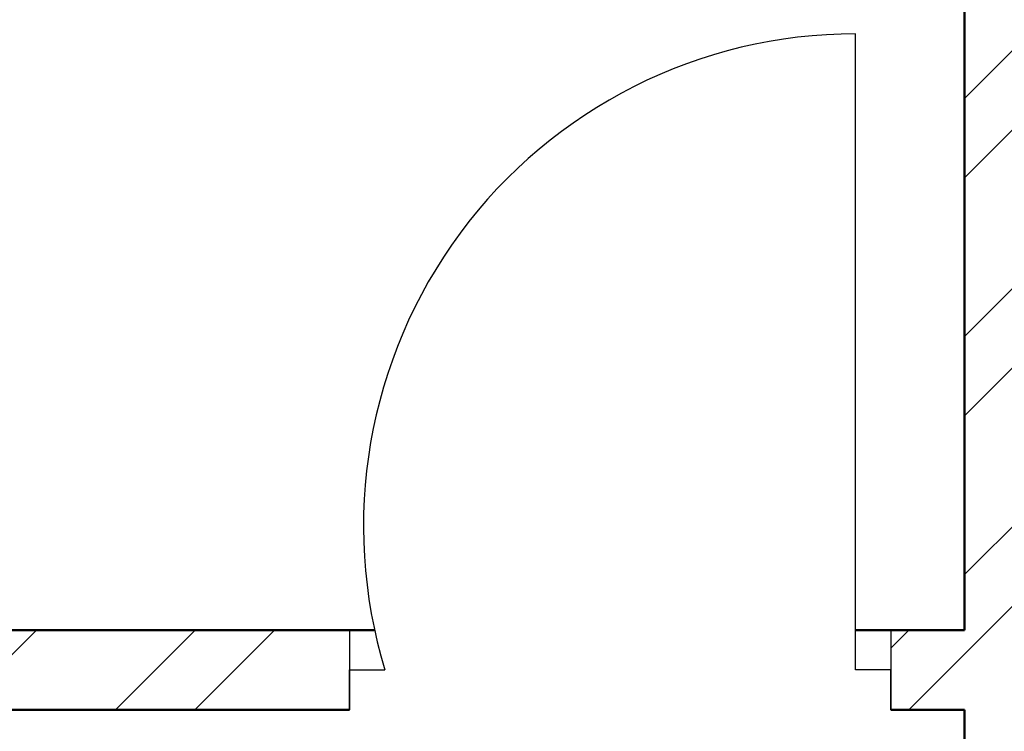
# Model space of a CAD drawing. Units: inches. Extents: x 963 to 2075, y 289 to 2657.
# Tile 70 of 98: x 1455 to 1511, y 2160 to 2200. Entities that reach past the tile are written whole.
import ezdxf

# ---------------------------------------------------------------- set-up
doc = ezdxf.new("R2010")
doc.units = ezdxf.units.IN
for name, color, linetype, lineweight in [('A-DOOR', 4, 'Continuous', 25), ('A-WALL', 7, 'Continuous', 50), ('A-WALL-PATT', 8, 'Continuous', 13)]:
    doc.layers.add(name, color=color, linetype=linetype, lineweight=lineweight)

msp = doc.modelspace()

# ---------------------------------------------------------------- hatches: boundary and pattern name
at = {"layer": 'A-WALL-PATT'}
h = msp.add_hatch(dxfattribs=at)
h.set_pattern_fill('ANSI32', color=256)
h.paths.add_polyline_path([(1296.922, 2558.318), (1203.922, 2558.318), (1203.922, 2493.818), (1191.533, 2493.818), (1191.533, 2489.318), (1211.063, 2489.318), (1211.063, 2492.02), (1211.063, 2493.818), (1208.422, 2493.818), (1208.422, 2553.818), (1292.422, 2553.818), (1292.422, 2538.863), (1296.922, 2538.863)])
h.paths.add_polyline_path([(1442.422, 2558.318), (1349.422, 2558.318), (1349.422, 2538.943), (1353.922, 2538.943), (1353.922, 2553.818), (1437.922, 2553.818), (1437.922, 2493.818), (1434.542, 2493.818), (1434.542, 2489.318), (1448.311, 2489.318), (1448.311, 2491.568), (1448.311, 2493.818), (1442.422, 2493.818)])
h.paths.add_polyline_path([(1415.554, 2491.568), (1415.554, 2493.818), (1340.941, 2493.818), (1340.941, 2489.318), (1371.922, 2489.318), (1371.922, 2378.318), (1367.596, 2378.318), (1367.596, 2373.818), (1371.922, 2373.818), (1371.922, 2355.185), (1376.422, 2355.185), (1376.422, 2489.318), (1415.554, 2489.318)])
h.paths.add_polyline_path([(1304.941, 2491.568), (1304.941, 2493.818), (1296.922, 2493.818), (1296.922, 2514.863), (1292.422, 2514.863), (1292.422, 2493.818), (1232.808, 2493.818), (1232.808, 2489.318), (1256.422, 2489.318), (1256.422, 2327.318), (1253.714, 2327.318), (1253.714, 2322.818), (1328.422, 2322.818), (1328.422, 2331.147), (1323.922, 2331.147), (1323.922, 2327.318), (1260.922, 2327.318), (1260.922, 2373.818), (1323.922, 2373.818), (1323.922, 2357.812), (1328.422, 2357.812), (1328.422, 2373.818), (1346.007, 2373.818), (1346.007, 2376.068), (1346.007, 2378.318), (1260.922, 2378.318), (1260.922, 2489.318), (1304.941, 2489.318)])
h.paths.add_polyline_path([(1226.654, 2327.318), (1124.422, 2327.318), (1124.422, 2347.447), (1119.922, 2347.447), (1119.922, 2322.818), (1163.422, 2322.818), (1163.422, 2305.435), (1165.672, 2305.435), (1167.922, 2305.435), (1167.922, 2322.818), (1226.654, 2322.818), (1226.654, 2325.068)])
h.paths.add_polyline_path([(1095.922, 2489.318), (1124.422, 2489.318), (1131.533, 2489.318), (1131.533, 2491.568), (1131.533, 2493.818), (1119.922, 2493.818), (1091.422, 2493.818), (1091.422, 2417.318), (1095.922, 2417.318), (1119.922, 2417.318), (1119.922, 2407.447), (1124.422, 2407.447), (1124.422, 2421.818), (1095.922, 2421.818)])
h.paths.add_polyline_path([(1512.922, 2558.318), (1508.422, 2558.318), (1508.422, 2493.818), (1503.401, 2493.818), (1503.401, 2489.318), (1508.422, 2489.318), (1508.422, 2327.318), (1376.422, 2327.318), (1376.422, 2330.273), (1371.922, 2330.273), (1371.922, 2298.744), (1376.422, 2298.744), (1376.422, 2322.818), (1508.422, 2322.818), (1508.422, 2165.318), (1504.255, 2165.318), (1504.255, 2160.818), (1508.422, 2160.818), (1508.422, 2108.318), (1512.922, 2108.318), (1512.922, 2160.818), (1516.182, 2160.818), (1516.182, 2163.068), (1516.182, 2165.318), (1512.922, 2165.318), (1512.922, 2322.818), (1644.922, 2322.818), (1644.922, 2298.744), (1649.422, 2298.744), (1649.422, 2322.818), (1649.422, 2330.944), (1647.172, 2330.944), (1644.922, 2330.944), (1644.922, 2327.318), (1512.922, 2327.318), (1512.922, 2489.318), (1516.759, 2489.318), (1516.759, 2491.568), (1516.759, 2493.818), (1512.922, 2493.818)])
h.paths.add_polyline_path([(1671.922, 2558.318), (1578.922, 2558.318), (1578.922, 2493.818), (1573.526, 2493.818), (1573.526, 2489.318), (1586.537, 2489.318), (1586.537, 2491.568), (1586.537, 2493.818), (1583.422, 2493.818), (1583.422, 2553.818), (1667.422, 2553.818), (1667.422, 2541.109), (1671.922, 2541.109)])
h.paths.add_polyline_path([(1681.257, 2493.818), (1671.922, 2493.818), (1671.922, 2517.109), (1667.422, 2517.109), (1667.422, 2493.818), (1610.218, 2493.818), (1610.218, 2489.318), (1644.922, 2489.318), (1644.922, 2357.865), (1649.422, 2357.865), (1649.422, 2373.818), (1652.203, 2373.818), (1652.203, 2375.827), (1652.203, 2378.318), (1649.422, 2378.318), (1649.422, 2489.318), (1681.257, 2489.318), (1681.257, 2491.568)])
h.paths.add_polyline_path([(1821.922, 2558.318), (1728.922, 2558.318), (1728.922, 2541), (1733.422, 2541), (1733.422, 2553.818), (1817.422, 2553.818), (1817.422, 2493.818), (1813.507, 2493.818), (1813.507, 2489.318), (1830.078, 2489.318), (1830.078, 2491.568), (1830.078, 2493.818), (1821.922, 2493.818)])
h.paths.add_polyline_path([(1794.244, 2493.818), (1717.257, 2493.818), (1717.257, 2489.318), (1760.422, 2489.318), (1760.422, 2378.318), (1674.401, 2378.318), (1674.401, 2373.818), (1692.922, 2373.818), (1692.922, 2356.954), (1697.422, 2356.954), (1697.422, 2373.818), (1760.422, 2373.818), (1760.422, 2327.318), (1697.422, 2327.318), (1697.422, 2333.341), (1692.922, 2333.341), (1692.922, 2322.818), (1768.037, 2322.818), (1768.037, 2325.068), (1768.037, 2327.318), (1764.922, 2327.318), (1764.922, 2489.318), (1794.244, 2489.318)])
h.paths.add_polyline_path([(1733.422, 2517), (1728.922, 2517), (1728.922, 2493.818), (1733.422, 2493.818)], flags=17)
h.paths.add_polyline_path([(1929.922, 2493.818), (1890.078, 2493.818), (1890.078, 2489.318), (1896.922, 2489.318), (1925.422, 2489.318), (1925.422, 2421.818), (1896.922, 2421.818), (1896.922, 2408.318), (1901.422, 2408.318), (1901.422, 2417.318), (1925.422, 2417.318), (1929.922, 2417.318)])
h.paths.add_polyline_path([(1901.422, 2348.318), (1896.922, 2348.318), (1896.922, 2327.318), (1800.423, 2327.318), (1800.423, 2322.818), (1853.422, 2322.818), (1853.422, 2309.453), (1857.922, 2309.453), (1857.922, 2322.818), (1901.422, 2322.818)])
h.paths.add_polyline_path([(1857.922, 2249.453), (1853.422, 2249.453), (1853.422, 2214.818), (1686.309, 2214.818), (1686.309, 2210.318), (1853.422, 2210.318), (1853.422, 2202.134), (1857.922, 2202.134), (1857.922, 2210.318)])
h.paths.add_polyline_path([(1857.922, 2142.134), (1853.422, 2142.134), (1853.422, 2115.422), (1841.422, 2115.422), (1841.422, 2088.531), (1841.422, 2046.949), (1845.922, 2046.949), (1845.922, 2110.922), (1905.922, 2110.922), (1905.922, 2092.517), (1910.422, 2092.517), (1910.422, 2115.422), (1857.922, 2115.422)])
h.paths.add_polyline_path([(1532.436, 1482.342), (1573.456, 1482.342), (1573.456, 1501), (1532.436, 1501)], flags=9)
h.paths.add_polyline_path([(1438.658, 1486.302), (1479.678, 1486.302), (1479.678, 1504.96), (1438.658, 1504.96)], flags=9)
h.paths.add_polyline_path([(1411.215, 1365.308), (1659.139, 1365.308), (1659.139, 1402.401), (1411.215, 1402.401)], flags=9)
h.paths.add_polyline_path([(1185.671, 2296.298), (1248.16, 2296.298), (1248.16, 2314.955), (1185.671, 2314.955)], flags=9)
h.paths.add_polyline_path([(1177.31, 2187.35), (1216.15, 2187.35), (1216.15, 2206.007), (1177.31, 2206.007)], flags=9)
h.paths.add_polyline_path([(1295.101, 1602.083), (1328.26, 1602.083), (1328.26, 1620.741), (1295.101, 1620.741)], flags=9)
h.paths.add_polyline_path([(1525.126, 2005.99), (1558.39, 2005.99), (1558.39, 2024.648), (1525.126, 2024.648)], flags=9)
h.paths.add_polyline_path([(1459.606, 1977.125), (1472.195, 1977.125), (1472.195, 1987.429), (1459.606, 1987.429)], flags=9)
h.paths.add_polyline_path([(1467.815, 2053.676), (1480.018, 2053.676), (1480.018, 2063.979), (1467.815, 2063.979)], flags=9)
h.paths.add_polyline_path([(1555.184, 2119.02), (1584.563, 2119.02), (1584.563, 2137.678), (1555.184, 2137.678)], flags=25)
h.paths.add_polyline_path([(1405.389, 2115.291), (1444.478, 2115.291), (1444.478, 2133.948), (1405.389, 2133.948)], flags=25)
h.paths.add_polyline_path([(1698.482, 2004.259), (1727.695, 2004.259), (1727.695, 2022.916), (1698.482, 2022.916)], flags=9)
h.paths.add_polyline_path([(1612.158, 1972.855), (1629.016, 1972.855), (1629.016, 1983.159), (1612.158, 1983.159)], flags=9)
h.paths.add_polyline_path([(1608.289, 2060.036), (1625.147, 2060.036), (1625.147, 2070.34), (1608.289, 2070.34)], flags=9)
h.paths.add_polyline_path([(1527.954, 1684.402), (1566.795, 1684.402), (1566.795, 1703.06), (1527.954, 1703.06)], flags=9)
h.paths.add_polyline_path([(1422.792, 1683.59), (1461.633, 1683.59), (1461.633, 1702.247), (1422.792, 1702.247)], flags=9)
h.paths.add_polyline_path([(1531.262, 1732.459), (1574.015, 1732.459), (1574.015, 1751.116), (1531.262, 1751.116)], flags=9)
h.paths.add_polyline_path([(1402.872, 1732.845), (1439.799, 1732.845), (1439.799, 1751.502), (1402.872, 1751.502)], flags=9)
h.paths.add_polyline_path([(1243.122, 1923.132), (1281.962, 1923.132), (1281.962, 1941.79), (1243.122, 1941.79)], flags=9)
h.paths.add_polyline_path([(1181.752, 1792.268), (1244.241, 1792.268), (1244.241, 1810.926), (1181.752, 1810.926)], flags=9)
h.paths.add_polyline_path([(1265.822, 1670.3), (1316.071, 1670.3), (1316.071, 1688.957), (1265.822, 1688.957)], flags=9)
h.paths.add_polyline_path([(1140.263, 1676.054), (1179.104, 1676.054), (1179.104, 1694.711), (1140.263, 1694.711)], flags=9)
h.paths.add_polyline_path([(1107.49, 1490.889), (1143.374, 1490.889), (1143.374, 1509.546), (1107.49, 1509.546)], flags=9)
h.paths.add_polyline_path([(1217.584, 1483.899), (1246.741, 1483.899), (1246.741, 1502.556), (1217.584, 1502.556)], flags=9)
h.paths.add_polyline_path([(1389.21, 1486.919), (1418.367, 1486.919), (1418.367, 1505.576), (1389.21, 1505.576)], flags=9)
h.paths.add_polyline_path([(1672.208, 1602.083), (1705.366, 1602.083), (1705.366, 1620.741), (1672.208, 1620.741)], flags=9)
h.paths.add_polyline_path([(1752.082, 1522.638), (1781.24, 1522.638), (1781.24, 1541.295), (1752.082, 1541.295)], flags=9)
h.paths.add_polyline_path([(1848.275, 1491.26), (1884.158, 1491.26), (1884.158, 1509.918), (1848.275, 1509.918)], flags=9)
h.paths.add_polyline_path([(1822.47, 1685.62), (1861.31, 1685.62), (1861.31, 1704.278), (1822.47, 1704.278)], flags=9)
h.paths.add_polyline_path([(1713.195, 1672.232), (1763.444, 1672.232), (1763.444, 1690.889), (1713.195, 1690.889)], flags=9)
h.paths.add_polyline_path([(1736.619, 1790.578), (1799.109, 1790.578), (1799.109, 1809.235), (1736.619, 1809.235)], flags=9)
h.paths.add_polyline_path([(1691.491, 1916.355), (1730.332, 1916.355), (1730.332, 1935.013), (1691.491, 1935.013)], flags=9)
h.paths.add_polyline_path([(1764.872, 1973.922), (1794.306, 1973.922), (1794.306, 1992.58), (1764.872, 1992.58)], flags=9)
h.paths.add_polyline_path([(1767.854, 2034.017), (1797.288, 2034.017), (1797.288, 2052.674), (1767.854, 2052.674)], flags=9)
h.paths.add_polyline_path([(1851.593, 2060.331), (1880.751, 2060.331), (1880.751, 2078.989), (1851.593, 2078.989)], flags=25)
h.paths.add_polyline_path([(1688.491, 2086.874), (1727.332, 2086.874), (1727.332, 2105.531), (1688.491, 2105.531)], flags=9)
h.paths.add_polyline_path([(1537.743, 2293.581), (1580.495, 2293.581), (1580.495, 2312.239), (1537.743, 2312.239)], flags=25)
h.paths.add_polyline_path([(1425.587, 2296.109), (1468.34, 2296.109), (1468.34, 2314.766), (1425.587, 2314.766)], flags=25)
h.paths.add_polyline_path([(1278.518, 2004.184), (1307.72, 2004.184), (1307.72, 2022.841), (1278.518, 2022.841)], flags=9)
h.paths.add_polyline_path([(1193.282, 1973.635), (1222.715, 1973.635), (1222.715, 1992.292), (1193.282, 1992.292)], flags=9)
h.paths.add_polyline_path([(1192.411, 2040.577), (1221.845, 2040.577), (1221.845, 2059.234), (1192.411, 2059.234)], flags=9)
h.paths.add_polyline_path([(1130.603, 1951.393), (1159.76, 1951.393), (1159.76, 1970.05), (1130.603, 1970.05)], flags=9)
h.paths.add_polyline_path([(1132.827, 2052.494), (1161.984, 2052.494), (1161.984, 2071.151), (1132.827, 2071.151)], flags=9)
h.paths.add_polyline_path([(1265.128, 2334.619), (1315.377, 2334.619), (1315.377, 2353.277), (1265.128, 2353.277)], flags=25)
h.paths.add_polyline_path([(1136.741, 2330.785), (1175.582, 2330.785), (1175.582, 2349.443), (1136.741, 2349.443)], flags=9)
h.paths.add_polyline_path([(1287.422, 2417.204), (1320.58, 2417.204), (1320.58, 2435.861), (1287.422, 2435.861)], flags=25)
h.paths.add_polyline_path([(1430.988, 2329.159), (1469.828, 2329.159), (1469.828, 2347.816), (1430.988, 2347.816)], flags=25)
h.paths.add_polyline_path([(1525.424, 2329.213), (1564.264, 2329.213), (1564.264, 2347.87), (1525.424, 2347.87)], flags=25)
h.paths.add_polyline_path([(1684.525, 2382.799), (1717.683, 2382.799), (1717.683, 2401.457), (1684.525, 2401.457)], flags=25)
h.paths.add_polyline_path([(1704.805, 2340.293), (1755.054, 2340.293), (1755.054, 2358.95), (1704.805, 2358.95)], flags=25)
h.paths.add_polyline_path([(1694.113, 2287.757), (1756.602, 2287.757), (1756.602, 2306.414), (1694.113, 2306.414)], flags=9)
h.paths.add_polyline_path([(1815.778, 2329.861), (1854.618, 2329.861), (1854.618, 2348.518), (1815.778, 2348.518)], flags=9)
h.paths.add_polyline_path([(1842.873, 2514.256), (1878.756, 2514.256), (1878.756, 2532.914), (1842.873, 2532.914)], flags=9)
h.paths.add_polyline_path([(1769.513, 2531.447), (1798.671, 2531.447), (1798.671, 2550.104), (1769.513, 2550.104)], flags=25)
h.paths.add_polyline_path([(1594.772, 2518.468), (1623.93, 2518.468), (1623.93, 2537.125), (1594.772, 2537.125)], flags=25)
h.paths.add_polyline_path([(1520.723, 2516.185), (1556.606, 2516.185), (1556.606, 2534.842), (1520.723, 2534.842)], flags=25)
h.paths.add_polyline_path([(1464.456, 2516.694), (1500.34, 2516.694), (1500.34, 2535.351), (1464.456, 2535.351)], flags=25)
h.paths.add_polyline_path([(1365.696, 2528.97), (1394.854, 2528.97), (1394.854, 2547.627), (1365.696, 2547.627)], flags=25)
h.paths.add_polyline_path([(1222.838, 2516.231), (1251.995, 2516.231), (1251.995, 2534.889), (1222.838, 2534.889)], flags=25)
h.paths.add_polyline_path([(1104.545, 2509.6), (1140.429, 2509.6), (1140.429, 2528.257), (1104.545, 2528.257)], flags=9)
h = msp.add_hatch(dxfattribs=at)
h.set_pattern_fill('ANSI32', color=256)
h.paths.add_polyline_path([(1473.609, 2163.068), (1473.609, 2165.318), (1376.422, 2165.318), (1376.422, 2227.983), (1371.922, 2227.983), (1371.922, 2214.818), (1368.405, 2214.818), (1368.405, 2210.318), (1371.922, 2210.318), (1371.922, 2160.818), (1395.922, 2160.818), (1395.922, 2090.318), (1217.345, 2090.318), (1217.345, 2085.818), (1395.922, 2085.818), (1458.922, 2085.818), (1458.922, 2108.318), (1454.422, 2108.318), (1454.422, 2090.318), (1400.422, 2090.318), (1400.422, 2160.818), (1473.609, 2160.818)])
h.paths.add_polyline_path([(1649.422, 2210.318), (1653.225, 2210.318), (1653.225, 2214.818), (1649.422, 2214.818), (1649.422, 2227.983), (1644.922, 2227.983), (1644.922, 2165.318), (1550.099, 2165.318), (1550.099, 2160.818), (1620.922, 2160.818), (1620.922, 2112.818), (1555.446, 2112.818), (1555.446, 2108.318), (1584.327, 2108.318), (1584.327, 2084.916), (1588.827, 2084.916), (1588.827, 2108.318), (1625.422, 2108.318), (1667.951, 2108.318), (1667.951, 2022.667), (1588.827, 2022.667), (1588.827, 2047.408), (1584.327, 2047.408), (1584.327, 1996.003), (1588.827, 1996.003), (1588.827, 2018.318), (1667.951, 2018.167), (1667.951, 1928.318), (1625.422, 1928.318), (1625.422, 1923.818), (1672.451, 1923.818), (1672.451, 1928.318), (1672.451, 1946.663), (1785.446, 1946.663), (1785.446, 1951.163), (1743.034, 1951.163), (1743.034, 2017.922), (1841.422, 2017.922), (1841.422, 2014.775), (1845.922, 2014.775), (1845.922, 2017.922), (1905.922, 2017.922), (1905.922, 1987.511), (1910.422, 1987.511), (1910.422, 2022.422), (1910.422, 2068.517), (1905.922, 2068.517), (1905.922, 2022.422), (1845.922, 2022.422), (1845.922, 2025.851), (1843.672, 2025.851), (1841.422, 2025.851), (1841.422, 2022.422), (1743.034, 2022.422), (1743.034, 2084.031), (1768.451, 2084.031), (1785.446, 2084.031), (1785.446, 2088.531), (1672.451, 2088.531), (1672.451, 2112.818), (1667.951, 2112.818), (1625.422, 2112.818), (1625.422, 2160.818), (1649.422, 2160.818)])
h.paths.add_polyline_path([(1672.451, 2084.031), (1738.534, 2084.031), (1738.534, 1951.163), (1672.451, 1951.163)], flags=16)
h.paths.add_polyline_path([(1672.451, 2084.031), (1738.534, 2084.031), (1705.492, 2017.597)], flags=0)
h.paths.add_polyline_path([(1262.766, 2085.818), (1258.266, 2085.818), (1258.266, 2023.278), (1184.422, 2023.278), (1184.422, 2018.778), (1258.266, 2018.778), (1258.266, 1950.818), (1262.766, 1950.818)])
h.paths.add_polyline_path([(1312.266, 2085.818), (1307.766, 2085.818), (1307.766, 1950.818), (1312.266, 1950.818)])
h.paths.add_polyline_path([(1458.922, 1950.818), (1395.922, 1950.818), (1216.568, 1950.818), (1216.568, 1946.318), (1346.422, 1946.318), (1395.922, 1946.318), (1395.922, 1875.818), (1371.922, 1875.818), (1371.922, 1826.318), (1368.931, 1826.318), (1368.931, 1821.818), (1371.922, 1821.818), (1371.922, 1813.622), (1376.422, 1813.622), (1376.422, 1871.318), (1474.504, 1871.318), (1474.504, 1873.568), (1474.504, 1875.818), (1400.422, 1875.818), (1400.422, 1946.318), (1454.422, 1946.318), (1454.422, 1928.318), (1458.922, 1928.318)])
h.paths.add_polyline_path([(1184.422, 2120.778), (1167.922, 2120.778), (1167.922, 2134.812), (1165.672, 2134.812), (1163.422, 2134.812), (1163.422, 2120.778), (1119.922, 2120.778), (1119.922, 2098.095), (1124.422, 2098.095), (1124.422, 2116.278), (1167.922, 2116.278), (1179.922, 2116.278), (1179.922, 2045.916), (1184.422, 2045.916), (1184.422, 2090.318), (1184.422, 2116.278)])
h.paths.add_polyline_path([(1124.422, 2018.778), (1179.922, 2018.778), (1179.922, 2016.294), (1184.422, 2016.294), (1184.422, 2023.278), (1184.422, 2026.588), (1182.172, 2026.588), (1179.922, 2026.588), (1179.922, 2023.278), (1124.422, 2023.278), (1124.422, 2074.095), (1119.922, 2074.095), (1119.922, 2018.778), (1119.922, 1979.633), (1124.422, 1979.633)])
h.paths.add_polyline_path([(1184.422, 1925.778), (1184.422, 1946.318), (1184.422, 1996.073), (1182.172, 1996.073), (1179.922, 1996.073), (1179.922, 1925.778), (1124.422, 1925.778), (1124.422, 1955.633), (1119.922, 1955.502), (1119.922, 1921.278), (1158.922, 1921.278), (1158.922, 1909.983), (1163.422, 1909.983), (1163.422, 1921.278), (1184.422, 1921.278)])
h.paths.add_polyline_path([(1341.449, 1826.318), (1163.422, 1826.318), (1163.422, 1849.983), (1158.922, 1849.983), (1158.922, 1821.818), (1158.922, 1804.033), (1163.422, 1804.033), (1163.422, 1821.818), (1341.449, 1821.818)])
h.paths.add_polyline_path([(1222.981, 1713.818), (1163.422, 1713.818), (1163.422, 1744.033), (1161.172, 1744.033), (1158.922, 1744.033), (1158.922, 1713.818), (1119.922, 1713.818), (1119.922, 1694.65), (1124.422, 1694.65), (1124.422, 1709.318), (1158.922, 1709.318), (1222.981, 1709.318)])
h.paths.add_polyline_path([(1328.422, 1713.818), (1252.042, 1713.818), (1252.042, 1711.568), (1252.042, 1709.318), (1256.422, 1709.318), (1256.422, 1547.318), (1232.937, 1547.318), (1232.937, 1545.068), (1232.937, 1542.818), (1292.422, 1542.818), (1292.422, 1527.634), (1296.922, 1527.634), (1296.922, 1542.818), (1299.464, 1542.818), (1299.464, 1547.318), (1260.922, 1547.318), (1260.922, 1658.318), (1343.661, 1658.318), (1343.661, 1660.568), (1343.661, 1662.818), (1328.422, 1662.818), (1328.422, 1676.589), (1327.402, 1676.589), (1323.922, 1676.589), (1323.922, 1662.818), (1260.922, 1662.818), (1260.922, 1709.318), (1323.922, 1709.318), (1323.922, 1699.851), (1328.422, 1699.851)])
h.paths.add_polyline_path([(1649.422, 1875.818), (1625.422, 1875.818), (1625.422, 1928.318), (1620.922, 1928.318), (1588.827, 1928.318), (1588.827, 1950.59), (1584.327, 1950.59), (1584.327, 1928.318), (1555.446, 1928.318), (1555.446, 1923.818), (1620.922, 1923.818), (1620.922, 1875.818), (1548.952, 1875.818), (1548.952, 1873.568), (1548.952, 1871.318), (1644.922, 1871.318), (1644.922, 1813.622), (1649.422, 1813.622), (1649.422, 1821.818), (1652.045, 1821.818), (1652.045, 1824.068), (1652.045, 1826.318), (1649.422, 1826.318)])
h.paths.add_polyline_path([(1512.922, 1871.318), (1516.476, 1871.318), (1516.476, 1875.818), (1512.922, 1875.818), (1512.922, 1923.818), (1512.922, 1928.318), (1512.922, 1930.827), (1508.422, 1930.827), (1508.422, 1875.818), (1504.411, 1875.818), (1504.411, 1871.318), (1508.422, 1871.318), (1508.422, 1713.818), (1376.422, 1713.818), (1376.422, 1743.325), (1371.922, 1743.325), (1371.922, 1709.318), (1371.922, 1706.01), (1376.422, 1706.01), (1376.422, 1709.318), (1508.422, 1709.318), (1508.422, 1547.318), (1501.871, 1547.318), (1501.871, 1542.818), (1508.422, 1542.818), (1508.422, 1482.818), (1508.422, 1436.318), (1512.922, 1436.318), (1512.922, 1542.818), (1519.318, 1542.818), (1519.318, 1545.068), (1519.318, 1547.318), (1512.922, 1547.318), (1512.922, 1709.318), (1644.922, 1709.318), (1644.922, 1707.548), (1649.422, 1707.548), (1649.422, 1709.318), (1649.422, 1743.325), (1644.922, 1743.325), (1644.922, 1713.818), (1512.922, 1713.818)])
h.paths.add_polyline_path([(1129.884, 1545.068), (1129.884, 1547.318), (1124.422, 1547.318), (1095.922, 1547.318), (1095.922, 1614.818), (1124.422, 1614.818), (1124.422, 1619.318), (1095.922, 1619.318), (1091.422, 1619.318), (1091.422, 1542.818), (1095.922, 1542.818), (1119.922, 1542.818), (1129.884, 1542.818)])
h.paths.add_polyline_path([(1208.422, 1542.818), (1211.74, 1542.818), (1211.74, 1547.318), (1198.851, 1547.318), (1198.851, 1542.818), (1203.922, 1542.818), (1203.922, 1478.318), (1208.422, 1478.318), (1296.922, 1478.318), (1296.922, 1503.634), (1292.422, 1503.634), (1292.422, 1482.818), (1208.422, 1482.818)])
h.paths.add_polyline_path([(1430.422, 1542.818), (1435.699, 1542.818), (1435.699, 1545.068), (1435.699, 1547.318), (1422.658, 1547.318), (1422.658, 1545.068), (1422.658, 1542.818), (1425.922, 1542.818), (1425.922, 1482.857), (1341.922, 1482.857), (1341.922, 1502.732), (1337.422, 1502.732), (1337.422, 1478.357), (1425.922, 1478.357), (1425.922, 1440.818), (1425.922, 1436.318), (1430.422, 1436.318)])
h.paths.add_polyline_path([(1698.482, 2004.259), (1727.695, 2004.259), (1727.695, 2022.916), (1698.482, 2022.916)], flags=8)

# ---------------------------------------------------------------- linework, layer by layer
at = {"layer": 'A-DOOR'}
for p, q in [((1502.255, 2163.068), (1502.255, 2199.068)), ((1473.609, 2165.318), (1473.609, 2160.818)), ((1504.255, 2165.318), (1504.255, 2160.818)), ((1473.609, 2160.818), (1473.609, 2163.068)), ((1473.609, 2163.068), (1475.609, 2163.068)), ((1504.255, 2163.068), (1502.255, 2163.068)), ((1504.255, 2160.818), (1504.255, 2163.068))]:
    msp.add_line(p, q, dxfattribs=at)
msp.add_arc((1502.255, 2171.206), 27.862, 90, 196.9833, dxfattribs=at)
at = {"layer": 'A-WALL'}
for p, q in [((1508.422, 2322.818), (1508.422, 2165.318)), ((1376.422, 2165.318), (1475.023, 2165.318)), ((1502.255, 2165.318), (1508.422, 2165.318)), ((1400.422, 2160.818), (1473.609, 2160.818)), ((1504.255, 2160.818), (1508.422, 2160.818)), ((1508.422, 2160.818), (1508.422, 2108.318))]:
    msp.add_line(p, q, dxfattribs=at)

doc.saveas('drawing.dxf')
